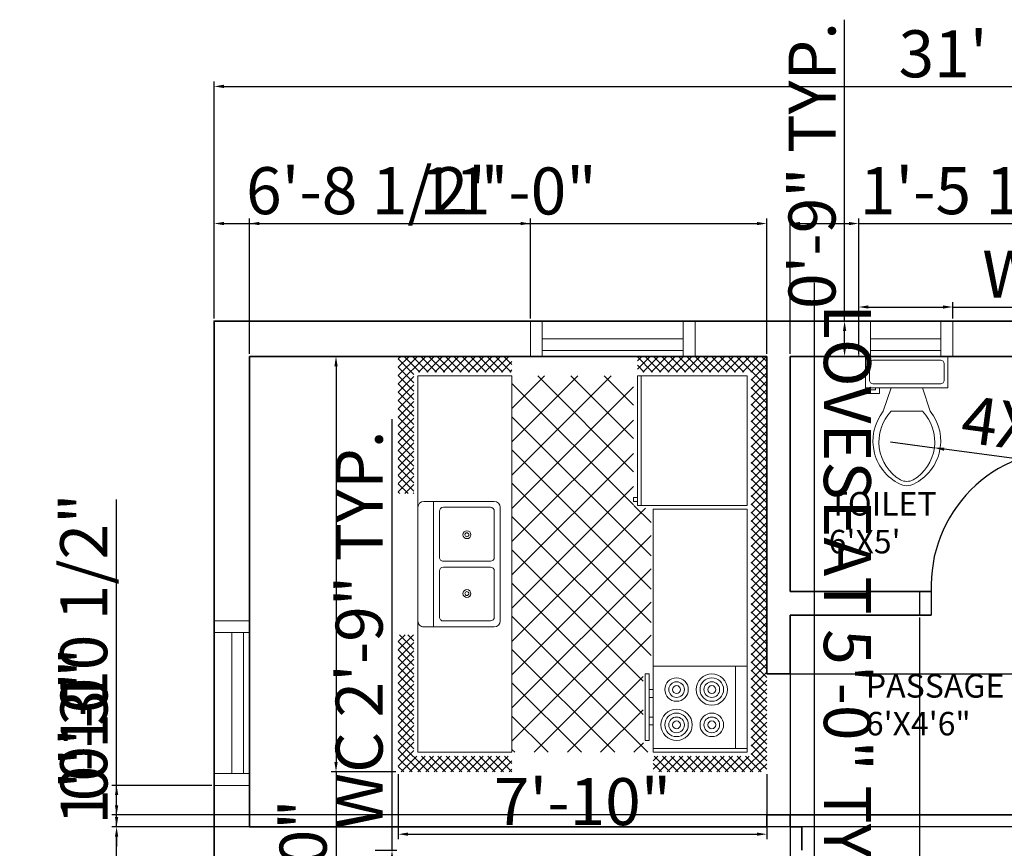
# Model space of a CAD drawing. Units: inches. Extents: x 2330 to 2931, y 514 to 1098.
# Tile 2 of 4: x 2332 to 2583, y 887 to 1098. Entities that reach past the tile are written whole.
import ezdxf

# ---------------------------------------------------------------- set-up
doc = ezdxf.new("R2010")
doc.units = ezdxf.units.IN
for name, color, linetype, lineweight in [('A-ANNO-DIMS', 2, 'Continuous', 18), ('A-AREA-IDEN', 7, 'Continuous', 18), ('A-DOOR', 3, 'Continuous', 25), ('A-FLOR-FIXT', 9, 'Continuous', 18), ('A-GLAZ', 4, 'Continuous', 18), ('A-WALL', 7, 'Continuous', 35)]:
    doc.layers.add(name, color=color, linetype=linetype, lineweight=lineweight)
doc.styles.get("Standard").update_dxf_attribs({"font": 'arial.ttf'})
doc.dimstyles.new('ISO-25', dxfattribs={"dimtxt": 12, "dimasz": 2.5, "dimexe": 1.25, "dimexo": 0.625, "dimtad": 1, "dimdec": 1, "dimlunit": 3, "dimtxsty": 'Standard', "dimcen": 2.5, "dimadec": 0, "dimazin": 0, "dimtfac": 1, "dimtdec": 1, "dimtmove": 0, "dimatfit": 3, "dimfxl": 1, "dimarcsym": 0})

# ---------------------------------------------------------------- blocks, each defined once
blk = doc.blocks.new('*D1')
at = {"layer": 'A-ANNO-DIMS', "color": 0, "lineweight": -2, "transparency": 16777216}
for p, q in [((2381.8, 1022.1), (2381.8, 1082.6)), ((2384.3, 1081.35), (2751.3, 1081.35)), ((2753.8, 1022.1), (2753.8, 1082.6))]:
    blk.add_line(p, q, dxfattribs=at)
at = {"layer": 'A-ANNO-DIMS', "color": 0, "transparency": 16777216}
for points in [[(2384.3, 1081.77), (2384.3, 1080.93), (2381.8, 1081.35)], [(2751.3, 1081.77), (2751.3, 1080.93), (2753.8, 1081.35)]]:
    blk.add_solid(points, dxfattribs=at)
at = {"layer": 'Defpoints', "color": 0, "transparency": 16777216}
for p in [(2753.8, 1081.35), (2381.8, 1021.47), (2753.8, 1021.47)]:
    blk.add_point(p, dxfattribs=at)
at = {"layer": 'A-ANNO-DIMS', "color": 0, "transparency": 16777216, "insert": (2567.8, 1088.11), "char_height": 12, "attachment_point": 5}
blk.add_mtext("31'", dxfattribs=at)
blk = doc.blocks.new('Kitchen Layout - 7 x 8 ft')
for p, q in [((-5, 81.32), (2.68, 89)), ((-5, 83.44), (0.56, 89)), ((-5, 85.56), (-1.56, 89)), ((-5, 87.68), (-3.68, 89)), ((-1, 84.97), (-5, 88.97)), ((1.09, 85), (-2.91, 89)), ((3.21, 85), (-0.79, 89)), ((0.81, 85), (4.81, 89)), ((5.34, 85), (1.34, 89)), ((2.93, 85), (6.93, 89)), ((7.46, 85), (3.46, 89)), ((5.05, 85), (9.05, 89)), ((9.58, 85), (5.58, 89)), ((7.17, 85), (11.17, 89)), ((11.7, 85), (7.7, 89)), ((9.29, 85), (13.29, 89)), ((13.82, 85), (9.82, 89)), ((11.41, 85), (15.41, 89)), ((15.94, 85), (11.94, 89)), ((13.53, 85), (17.53, 89)), ((18.06, 85), (14.06, 89)), ((15.65, 85), (19.65, 89)), ((20.18, 85), (16.18, 89)), ((17.78, 85), (21.78, 89)), ((22.31, 85), (18.31, 89)), ((19.9, 85), (23.9, 89)), ((24.43, 85), (20.43, 89)), ((22.02, 85), (26.02, 89)), ((26.55, 85), (22.55, 89)), ((24.14, 85), (28.14, 89)), ((28.67, 85), (24.67, 89)), ((26.26, 85), (30.26, 89)), ((30.79, 85), (26.79, 89)), ((28.38, 85), (32.38, 89)), ((32.91, 85), (28.91, 89)), ((30.5, 85), (34.5, 89)), ((35.03, 85), (31.03, 89)), ((32.63, 85), (36.63, 89)), ((37.16, 85), (33.16, 89)), ((34.75, 85), (38.75, 89)), ((39.28, 85), (35.28, 89)), ((36.87, 85), (40.87, 89)), ((41.4, 85), (37.4, 89)), ((38.99, 85), (42.99, 89)), ((43.52, 85), (39.52, 89)), ((41.11, 85), (45.11, 89)), ((45.64, 85), (41.64, 89)), ((43.23, 85), (47.23, 89)), ((47.76, 85), (43.76, 89)), ((45.35, 85), (49.35, 89)), ((49.88, 85), (45.88, 89)), ((47.47, 85), (51.47, 89)), ((52, 85), (48, 89)), ((49.6, 85), (53.6, 89)), ((54.13, 85), (50.13, 89)), ((51.72, 85), (55.72, 89)), ((56.25, 85), (52.25, 89)), ((53.84, 85), (57.84, 89)), ((58.37, 85), (54.37, 89)), ((55.96, 85), (59.96, 89)), ((60.49, 85), (56.49, 89)), ((58.08, 85), (62.08, 89)), ((62.61, 85), (58.61, 89)), ((60.2, 85), (64.2, 89)), ((64.73, 85), (60.73, 89)), ((62.32, 85), (66.32, 89)), ((66.85, 85), (62.85, 89)), ((64.45, 85), (68.45, 89)), ((68.97, 85), (64.97, 89)), ((66.57, 85), (70.57, 89)), ((71.1, 85), (67.1, 89)), ((68.69, 85), (72.69, 89)), ((73.22, 85), (69.22, 89)), ((70.81, 85), (74.81, 89)), ((75.34, 85), (71.34, 89)), ((72.93, 85), (76.93, 89)), ((77.46, 85), (73.46, 89)), ((75.05, 85), (79.05, 89)), ((79.58, 85), (75.58, 89)), ((77.17, 85), (81.17, 89)), ((81.7, 85), (77.7, 89)), ((79.29, 85), (83.29, 89)), ((83.82, 85), (79.82, 89)), ((81.42, 85), (85.42, 89)), ((85.95, 85), (81.95, 89)), ((83.54, 85), (87.54, 89)), ((88.07, 85), (84.07, 89)), ((85.66, 85), (89.66, 89)), ((90.19, 85), (86.19, 89)), ((87.78, 85), (91.78, 89)), ((92.31, 85), (88.31, 89)), ((89.9, 85), (93.9, 89)), ((94.43, 85), (90.43, 89)), ((92.02, 85), (96.02, 89)), ((96.55, 85), (92.55, 89)), ((94.14, 85), (98.14, 89)), ((101, 82.67), (94.67, 89)), ((96.27, 85), (100.27, 89)), ((101, 84.79), (96.79, 89)), ((101, 86.92), (98.92, 89)), ((-1, 82.85), (-5, 86.85)), ((97, 83.61), (101, 87.61)), ((97, 81.49), (101, 85.49)), ((-1, 80.73), (-5, 84.73)), ((-5, 79.19), (-1, 83.19)), ((34, 84), (96, 84)), ((34, 60), (34, 84)), ((96, 84), (96, 60)), ((101, 80.55), (97, 84.55)), ((97, 79.37), (101, 83.37)), ((-1, 78.61), (-5, 82.61)), ((-5, 77.07), (-1, 81.07)), ((-1, 76.49), (-5, 80.49)), ((74, 81), (95, 81)), ((101, 78.43), (97, 82.43)), ((97, 77.25), (101, 81.25)), ((-5, 74.95), (-1, 78.95)), ((-1, 74.36), (-5, 78.36)), ((101, 76.31), (97, 80.31)), ((97, 75.13), (101, 79.13)), ((101, 74.19), (97, 78.19)), ((-5, 72.83), (-1, 76.83)), ((-1, 72.24), (-5, 76.24)), ((97, 73.01), (101, 77.01)), ((101, 72.07), (97, 76.07)), ((-5, 70.71), (-1, 74.71)), ((-1, 70.12), (-5, 74.12)), ((97, 70.89), (101, 74.89)), ((101, 69.95), (97, 73.95)), ((-5, 68.59), (-1, 72.59)), ((-1, 68), (-5, 72)), ((-5, 66.47), (-1, 70.47)), ((97, 68.76), (101, 72.76)), ((101, 67.82), (97, 71.82)), ((97, 66.64), (101, 70.64)), ((-1, 65.88), (-5, 69.88)), ((-5, 64.35), (-1, 68.35)), ((101, 65.7), (97, 69.7)), ((97, 64.52), (101, 68.52)), ((-1, 63.76), (-5, 67.76)), ((-5, 62.22), (-1, 66.22)), ((-1, 61.64), (-5, 65.64)), ((101, 63.58), (97, 67.58)), ((97, 62.4), (101, 66.4)), ((101, 61.46), (97, 65.46)), ((-5, 60.1), (-1, 64.1)), ((-1, 59.52), (-5, 63.52)), ((97, 60.28), (101, 64.28)), ((100.34, 60), (97, 63.34)), ((-5, 57.98), (-1, 61.98)), ((-1, 57.39), (-5, 61.39)), ((98.22, 60), (97, 61.22)), ((98.84, 60), (101, 62.16)), ((-1.73, 56), (-5, 59.27)), ((-4.86, 56), (-1, 59.86)), ((10.4, 24), (45.9, 59.5)), ((18.88, 24), (54.38, 59.5)), ((27.37, 24), (62.87, 59.5)), ((33.03, 55.11), (37.41, 59.5)), ((67.71, 24), (33.68, 58.04)), ((96, 60), (34, 60)), ((35.85, 24), (71.35, 59.5)), ((76.2, 24), (40.7, 59.5)), ((84.68, 24), (49.18, 59.5)), ((93.17, 24), (57.67, 59.5)), ((61.31, 24), (96, 58.69)), ((96, 29.65), (66.15, 59.5)), ((80, 60), (80, 59)), ((82, 59), (82, 60)), ((87, 59), (87, 60)), ((89, 60), (89, 59)), ((100.96, 60), (101, 60.04)), ((-3.85, 56), (-5, 57.15)), ((-2.74, 56), (-1, 57.74)), ((0, 57), (33, 57)), ((31, 55), (31, 56)), ((32, 56), (32, 55)), ((44.34, 24), (77.84, 57.5)), ((52.82, 24), (86.32, 57.5)), ((96, 38.14), (76.64, 57.5)), ((96, 46.63), (85.13, 57.5)), ((96, 55.11), (93.57, 57.54)), ((0, 30.57), (24.43, 55)), ((0, 39.06), (15.94, 55)), ((0, 47.54), (7.46, 55)), ((1.91, 24), (32.91, 55)), ((33.77, 24), (2.77, 55)), ((42.26, 24), (11.26, 55)), ((50.74, 24), (19.74, 55)), ((59.23, 24), (28.23, 55)), ((32, 55), (31, 55)), ((25.29, 24), (0, 49.29)), ((69.79, 24), (96, 50.21)), ((16.8, 24), (0, 40.8)), ((78.28, 24), (96, 41.72)), ((86.76, 24), (96, 33.24)), ((8.32, 24), (0, 32.32)), ((-5, 21.92), (-2.92, 24)), ((-5, 19.8), (-1, 23.8)), ((-1, 19.21), (-5, 23.21)), ((-1, 21.33), (-3.67, 24)), ((-1, 23.45), (-1.55, 24)), ((0, 24), (96, 24)), ((0, 0), (0, 24)), ((95.25, 24), (96, 24.75)), ((96, 24), (96, 0)), ((97, 22.1), (98.9, 24)), ((97, 19.97), (101, 23.97)), ((101, 19.03), (97, 23.03)), ((101, 21.16), (98.16, 24)), ((101, 23.28), (100.28, 24)), ((-5, 17.68), (-1, 21.68)), ((-1, 17.09), (-5, 21.09)), ((97, 17.85), (101, 21.85)), ((101, 16.91), (97, 20.91)), ((-5, 15.55), (-1, 19.55)), ((-1, 14.97), (-5, 18.97)), ((47.25, 6.5), (47.25, 18.5)), ((48.75, 18.5), (48.75, 6.5)), ((97, 15.73), (101, 19.73)), ((101, 14.79), (97, 18.79)), ((97, 13.61), (101, 17.61)), ((-5, 13.43), (-1, 17.43)), ((-1, 12.85), (-5, 16.85)), ((-5, 11.31), (-1, 15.31)), ((101, 12.67), (97, 16.67)), ((97, 11.49), (101, 15.49)), ((-1, 10.73), (-5, 14.73)), ((-5, 9.19), (-1, 13.19)), ((-1, 8.6), (-5, 12.6)), ((101, 10.55), (97, 14.55)), ((97, 9.37), (101, 13.37)), ((-5, 7.07), (-1, 11.07)), ((-1, 6.48), (-5, 10.48)), ((101, 8.43), (97, 12.43)), ((97, 7.25), (101, 11.25)), ((101, 6.31), (97, 10.31)), ((-5, 4.95), (-1, 8.95)), ((-1, 4.36), (-5, 8.36)), ((97, 5.12), (101, 9.12)), ((101, 4.18), (97, 8.18)), ((-5, 2.83), (-1, 6.83)), ((-1, 2.24), (-5, 6.24)), ((97, 3), (101, 7)), ((101, 2.06), (97, 6.06)), ((-5, 0.71), (-1, 4.71)), ((-1, 0.12), (-5, 4.12)), ((-5, -1.42), (-1, 2.58)), ((64, 4), (32, 4)), ((93.24, -5), (101, 2.76)), ((97, 0.88), (101, 4.88)), ((101, -0.06), (97, 3.94)), ((2, -5), (-5, 2)), ((-5, -3.54), (-1, 0.46)), ((96, 0), (0, 0)), ((95.36, -5), (101, 0.64)), ((101, -2.18), (97, 1.82)), ((-0.12, -5), (-5, -0.12)), ((-2.25, -5), (-5, -2.25)), ((-4.34, -5), (-0.34, -1)), ((-2.22, -5), (1.78, -1)), ((-0.1, -5), (3.9, -1)), ((4.12, -5), (0.12, -1)), ((2.02, -5), (6.02, -1)), ((6.24, -5), (2.24, -1)), ((4.14, -5), (8.14, -1)), ((8.36, -5), (4.36, -1)), ((6.27, -5), (10.27, -1)), ((10.48, -5), (6.48, -1)), ((8.39, -5), (12.39, -1)), ((12.6, -5), (8.6, -1)), ((10.51, -5), (14.51, -1)), ((14.73, -5), (10.73, -1)), ((12.63, -5), (16.63, -1)), ((16.85, -5), (12.85, -1)), ((14.75, -5), (18.75, -1)), ((18.97, -5), (14.97, -1)), ((16.87, -5), (20.87, -1)), ((21.09, -5), (17.09, -1)), ((18.99, -5), (22.99, -1)), ((23.21, -5), (19.21, -1)), ((21.11, -5), (25.11, -1)), ((25.33, -5), (21.33, -1)), ((23.24, -5), (27.24, -1)), ((27.45, -5), (23.45, -1)), ((25.36, -5), (29.36, -1)), ((29.57, -5), (25.57, -1)), ((27.48, -5), (30, -2.48)), ((30, -3.3), (27.7, -1)), ((30, -1.18), (29.82, -1)), ((66, -2.54), (67.54, -1)), ((66, -4.66), (69.66, -1)), ((69.88, -5), (66, -1.12)), ((67.78, -5), (71.78, -1)), ((72, -5), (68, -1)), ((69.9, -5), (73.9, -1)), ((74.12, -5), (70.12, -1)), ((72.03, -5), (76.03, -1)), ((76.24, -5), (72.24, -1)), ((74.15, -5), (78.15, -1)), ((78.36, -5), (74.36, -1)), ((76.27, -5), (80.27, -1)), ((80.49, -5), (76.49, -1)), ((78.39, -5), (82.39, -1)), ((82.61, -5), (78.61, -1)), ((80.51, -5), (84.51, -1)), ((84.73, -5), (80.73, -1)), ((82.63, -5), (86.63, -1)), ((86.85, -5), (82.85, -1)), ((84.75, -5), (88.75, -1)), ((88.97, -5), (84.97, -1)), ((86.88, -5), (90.88, -1)), ((91.09, -5), (87.09, -1)), ((89, -5), (93, -1)), ((93.21, -5), (89.21, -1)), ((91.12, -5), (95.12, -1)), ((95.34, -5), (91.34, -1)), ((97.46, -5), (93.46, -1)), ((99.58, -5), (95.58, -1)), ((101, -4.3), (97, -0.3)), ((97.48, -5), (101, -1.48)), ((-4.37, -5), (-5, -4.37)), ((29.6, -5), (30, -4.6)), ((67.76, -5), (66, -3.24)), ((99.6, -5), (101, -3.6))]:
    blk.add_line(p, q)
for points in [[(0, 56), (0, 84), (33, 84), (33, 56)], [(74, 60), (74, 84), (95, 84), (95, 60)], [(76, 58), (76, 59), (93, 59), (93, 58)]]:
    blk.add_lwpolyline(points, close=True)
for points in [[(33.5, 21), (62.5, 21)], [(32, 1.5), (32, 19.5)], [(33.5, 6.5), (33.5, 18.5)], [(34.5, 19.5), (46.25, 19.5)], [(49.75, 19.5), (61.5, 19.5)], [(62.5, 18.5), (62.5, 6.5)], [(64, 19.5), (64, 1.5)], [(46.25, 5.5), (34.5, 5.5)], [(61.5, 5.5), (49.75, 5.5)], [(62.5, 0), (33.5, 0)]]:
    blk.add_lwpolyline(points)
for centre, radius in [((80, 75), 4), ((80, 75), 3), ((89, 75), 3), ((80, 75), 2), ((80, 75), 1), ((89, 75), 2), ((89, 75), 1), ((80, 66), 3), ((80, 66), 2), ((89, 66), 4), ((89, 66), 3), ((89, 66), 2), ((80, 66), 1), ((89, 66), 1), ((40.5, 12.5), 1), ((40.5, 12.5), 0.5), ((55.5, 12.5), 1), ((55.5, 12.5), 0.5)]:
    blk.add_circle(centre, radius)
for centre, radius, start, end in [((33.5, 19.5), 1.5, 90, 180), ((62.5, 19.5), 1.5, 0, 90), ((34.5, 18.5), 1, 90, 180), ((46.25, 18.5), 1, 0, 90), ((49.75, 18.5), 1, 90, 180), ((61.5, 18.5), 1, 0, 90), ((34.5, 6.5), 1, 180, 270), ((46.25, 6.5), 1, 270, 0), ((49.75, 6.5), 1, 180, 270), ((61.5, 6.5), 1, 270, 0), ((33.5, 1.5), 1.5, 180, 270), ((62.5, 1.5), 1.5, 270, 0)]:
    blk.add_arc(centre, radius, start, end)
blk = doc.blocks.new('Toilet - top')
for p, q in [((9.5, -6), (9.5, -2)), ((-10, -8.5), (-8, -8.5)), ((-10, -9.5), (-10, -8.5)), ((-7, -9.5), (-10, -9.5)), ((-8, -8.5), (-8, -8)), ((-7, -8), (-7, -9.5)), ((-4, -8), (-6, -14)), ((4, -8), (6, -14)), ((4, -14), (-4, -14))]:
    blk.add_line(p, q)
blk.add_lwpolyline([(10.5, -8), (10.5, 0), (-10.5, 0), (-10.5, -8)], close=True)
for points in [[(-9.5, -2), (-9.5, -6)], [(8.5, -1), (-8.5, -1)], [(-8.5, -7), (8.5, -7)]]:
    blk.add_lwpolyline(points)
for centre, radius, start, end in [((-8.62, -1.88), 0.884, 81.8699, 188.1301), ((8.62, -1.88), 0.884, 351.8699, 98.1301), ((-8.62, -6.12), 0.884, 171.8699, 278.1301), ((8.62, -6.12), 0.884, 261.8699, 8.1301), ((3.52, -21.58), 12.17, 141.4691, 247.9714), ((4.2, -21.82), 11.33, 136.3677, 238.9468), ((-3.52, -21.58), 12.17, 292.0284, 38.5307), ((-4.2, -21.82), 11.33, 301.053, 43.6321), ((0, -27.88), 4, 245.7318, 294.2682), ((0, -29), 4, 254.8605, 285.1395)]:
    blk.add_arc(centre, radius, start, end)
blk = doc.blocks.new('DOOR-SWING-36IN')
for p, q in [((0, 6), (0, 0)), ((3, 6), (3, 0)), ((39, 6), (39, 0)), ((42, 6), (42, 0))]:
    blk.add_line(p, q)
blk.add_lwpolyline([(39, 6), (36, 6), (36, 42), (39, 42)], close=True)
blk.add_arc((37.5, 7.5), 34.53, 87.5104, 182.4896)
blk = doc.blocks.new('WIN-36IN')
for p, q in [((0, 9), (0, 0)), ((39, 9), (3, 9)), ((3, 9), (3, 0)), ((39, 0), (39, 9)), ((42, 0), (42, 9)), ((3, 4.5), (39, 4.5)), ((3, 1.5), (39, 1.5)), ((3, 0), (39, 0))]:
    blk.add_line(p, q)
blk = doc.blocks.new('WIN-18IN')
for p, q in [((0, 9), (0, 0)), ((21, 9), (3, 9)), ((3, 9), (3, 0)), ((21, 0), (21, 9)), ((24, 0), (24, 9)), ((3, 4.5), (21, 4.5)), ((3, 1.5), (21, 1.5)), ((3, 0), (21, 0))]:
    blk.add_line(p, q)
blk = doc.blocks.new('*D19')
at = {"layer": 'A-ANNO-DIMS', "color": 0, "lineweight": -2, "transparency": 16777216}
for p, q in [((2546.27, 1022.1), (2546.27, 1026.32)), ((2570.27, 1022.1), (2570.27, 1026.32)), ((2548.77, 1025.07), (2567.77, 1025.07)), ((2570.27, 1025.07), (2755.68, 1025.07))]:
    blk.add_line(p, q, dxfattribs=at)
at = {"layer": 'A-ANNO-DIMS', "color": 0, "transparency": 16777216}
for points in [[(2548.77, 1025.49), (2548.77, 1024.66), (2546.27, 1025.07)], [(2567.77, 1025.49), (2567.77, 1024.66), (2570.27, 1025.07)]]:
    blk.add_solid(points, dxfattribs=at)
at = {"layer": 'Defpoints', "color": 0, "transparency": 16777216}
for p in [(2570.27, 1025.07), (2546.27, 1021.47), (2570.27, 1021.47)]:
    blk.add_point(p, dxfattribs=at)
at = {"layer": 'A-ANNO-DIMS', "color": 0, "transparency": 16777216, "insert": (2664.23, 1031.91), "char_height": 12, "attachment_point": 5}
blk.add_mtext('WINDOW W2 2\'-0" TYP.', dxfattribs=at)
blk = doc.blocks.new('*D20')
at = {"layer": 'A-ANNO-DIMS', "color": 0, "lineweight": -2, "transparency": 16777216}
for p, q in [((2542.67, 1021.47), (2542.67, 1098.37)), ((2545.65, 1021.47), (2541.42, 1021.47)), ((2542.67, 1014.97), (2542.67, 1018.97)), ((2545.65, 1012.47), (2541.42, 1012.47))]:
    blk.add_line(p, q, dxfattribs=at)
at = {"layer": 'A-ANNO-DIMS', "color": 0, "transparency": 16777216}
for points in [[(2542.26, 1018.97), (2543.09, 1018.97), (2542.67, 1021.47)], [(2542.26, 1014.97), (2543.09, 1014.97), (2542.67, 1012.47)]]:
    blk.add_solid(points, dxfattribs=at)
at = {"layer": 'Defpoints', "color": 0, "transparency": 16777216}
for p in [(2542.67, 1021.47), (2546.27, 1021.47), (2546.27, 1012.47)]:
    blk.add_point(p, dxfattribs=at)
at = {"layer": 'A-ANNO-DIMS', "color": 0, "transparency": 16777216, "insert": (2535.92, 1061.17), "char_height": 12, "attachment_point": 5, "rotation": 90}
blk.add_mtext('0\'-9" TYP.', dxfattribs=at)
blk = doc.blocks.new('*D23')
at = {"layer": 'A-ANNO-DIMS', "color": 0, "lineweight": -2, "transparency": 16777216}
for p, q in [((2427.19, 886.47), (2427.19, 996.45)), ((2422.86, 886.47), (2428.44, 886.47)), ((2427.19, 855.93), (2427.19, 883.97)), ((2422.86, 853.43), (2428.44, 853.43))]:
    blk.add_line(p, q, dxfattribs=at)
at = {"layer": 'A-ANNO-DIMS', "color": 0, "transparency": 16777216}
for points in [[(2426.77, 883.97), (2427.61, 883.97), (2427.19, 886.47)], [(2426.77, 855.93), (2427.61, 855.93), (2427.19, 853.43)]]:
    blk.add_solid(points, dxfattribs=at)
at = {"layer": 'Defpoints', "color": 0, "transparency": 16777216}
for p in [(2422.23, 886.47), (2427.19, 886.47), (2422.23, 853.43)]:
    blk.add_point(p, dxfattribs=at)
at = {"layer": 'A-ANNO-DIMS', "color": 0, "transparency": 16777216, "insert": (2420.36, 942.71), "char_height": 12, "attachment_point": 5, "rotation": 90}
blk.add_mtext('WC 2\'-9" TYP.', dxfattribs=at)
blk = doc.blocks.new('*D25')
at = {"layer": 'A-ANNO-DIMS', "color": 0, "lineweight": -2, "transparency": 16777216}
for p, q in [((2535, 861.7), (2535, 1031.23)), ((2543.37, 861.7), (2533.75, 861.7)), ((2535, 804.2), (2535, 859.2)), ((2543.37, 801.7), (2533.75, 801.7))]:
    blk.add_line(p, q, dxfattribs=at)
at = {"layer": 'A-ANNO-DIMS', "color": 0, "transparency": 16777216}
for points in [[(2535.41, 859.2), (2534.58, 859.2), (2535, 861.7)], [(2535.41, 804.2), (2534.58, 804.2), (2535, 801.7)]]:
    blk.add_solid(points, dxfattribs=at)
at = {"layer": 'Defpoints', "color": 0, "transparency": 16777216}
for p in [(2535, 861.7), (2544, 861.7), (2544, 801.7)]:
    blk.add_point(p, dxfattribs=at)
at = {"layer": 'A-ANNO-DIMS', "color": 0, "transparency": 16777216, "insert": (2541.83, 947.72), "char_height": 12, "attachment_point": 5, "rotation": 270.0001}
blk.add_mtext('LOVESEAT 5\'-0" TYP.', dxfattribs=at)
blk = doc.blocks.new('*D31')
at = {"layer": 'A-ANNO-DIMS', "color": 0, "lineweight": -2, "transparency": 16777216}
for p, q in [((2428.18, 1012.47), (2411.65, 1012.47)), ((2412.9, 1009.97), (2412.9, 908.97)), ((2428.18, 906.47), (2411.65, 906.47)), ((2412.9, 906.47), (2412.9, 712.06))]:
    blk.add_line(p, q, dxfattribs=at)
at = {"layer": 'A-ANNO-DIMS', "color": 0, "transparency": 16777216}
for points in [[(2412.49, 1009.97), (2413.32, 1009.97), (2412.9, 1012.47)], [(2412.49, 908.97), (2413.32, 908.97), (2412.9, 906.47)]]:
    blk.add_solid(points, dxfattribs=at)
at = {"layer": 'Defpoints', "color": 0, "transparency": 16777216}
for p in [(2428.8, 1012.47), (2412.9, 906.47), (2428.8, 906.47)]:
    blk.add_point(p, dxfattribs=at)
at = {"layer": 'A-ANNO-DIMS', "color": 0, "transparency": 16777216, "insert": (2406.07, 808.02), "char_height": 12, "attachment_point": 5, "rotation": 90}
blk.add_mtext('KITCHEN LAYOUT 8\'-10"', dxfattribs=at)
blk = doc.blocks.new('*D32')
at = {"layer": 'A-ANNO-DIMS', "color": 0, "lineweight": -2, "transparency": 16777216}
for p, q in [((2428.8, 905.85), (2428.8, 889.32)), ((2522.8, 905.85), (2522.8, 889.32)), ((2431.3, 890.57), (2520.3, 890.57))]:
    blk.add_line(p, q, dxfattribs=at)
at = {"layer": 'A-ANNO-DIMS', "color": 0, "transparency": 16777216}
for points in [[(2431.3, 890.99), (2431.3, 890.16), (2428.8, 890.57)], [(2520.3, 890.99), (2520.3, 890.16), (2522.8, 890.57)]]:
    blk.add_solid(points, dxfattribs=at)
at = {"layer": 'Defpoints', "color": 0, "transparency": 16777216}
for p in [(2428.8, 906.47), (2522.8, 906.47), (2522.8, 890.57)]:
    blk.add_point(p, dxfattribs=at)
at = {"layer": 'A-ANNO-DIMS', "color": 0, "transparency": 16777216, "insert": (2475.8, 897.32), "char_height": 12, "attachment_point": 5}
blk.add_mtext('7\'-10"', dxfattribs=at)
blk = doc.blocks.new('*D37')
at = {"layer": 'A-ANNO-DIMS', "color": 0, "lineweight": -2, "transparency": 16777216}
for p, q in [((2390.8, 1013.1), (2390.8, 1047.61)), ((2393.3, 1046.36), (2520.3, 1046.36)), ((2522.8, 1013.1), (2522.8, 1047.61))]:
    blk.add_line(p, q, dxfattribs=at)
at = {"layer": 'A-ANNO-DIMS', "color": 0, "transparency": 16777216}
for points in [[(2393.3, 1046.78), (2393.3, 1045.95), (2390.8, 1046.36)], [(2520.3, 1046.78), (2520.3, 1045.95), (2522.8, 1046.36)]]:
    blk.add_solid(points, dxfattribs=at)
at = {"layer": 'Defpoints', "color": 0, "transparency": 16777216}
for p in [(2522.8, 1046.36), (2390.8, 1012.47), (2522.8, 1012.47)]:
    blk.add_point(p, dxfattribs=at)
at = {"layer": 'A-ANNO-DIMS', "color": 0, "transparency": 16777216, "insert": (2456.8, 1053.12), "char_height": 12, "attachment_point": 5}
blk.add_mtext('11\'-0"', dxfattribs=at)
blk = doc.blocks.new('*D38')
at = {"layer": 'A-ANNO-DIMS', "color": 0, "lineweight": -2, "transparency": 16777216}
for p, q in [((2381.8, 1022.1), (2381.8, 1047.61)), ((2384.3, 1046.36), (2460.01, 1046.36)), ((2462.51, 1022.1), (2462.51, 1047.61))]:
    blk.add_line(p, q, dxfattribs=at)
at = {"layer": 'A-ANNO-DIMS', "color": 0, "transparency": 16777216}
for points in [[(2384.3, 1046.78), (2384.3, 1045.95), (2381.8, 1046.36)], [(2460.01, 1046.78), (2460.01, 1045.95), (2462.51, 1046.36)]]:
    blk.add_solid(points, dxfattribs=at)
at = {"layer": 'Defpoints', "color": 0, "transparency": 16777216}
for p in [(2462.51, 1046.36), (2381.8, 1021.47), (2462.51, 1021.47)]:
    blk.add_point(p, dxfattribs=at)
at = {"layer": 'A-ANNO-DIMS', "color": 0, "transparency": 16777216, "insert": (2422.16, 1053.19), "char_height": 12, "attachment_point": 5}
blk.add_mtext('6\'-8 1/2"', dxfattribs=at)
blk = doc.blocks.new('*D40')
at = {"layer": 'A-ANNO-DIMS', "color": 0, "lineweight": -2, "transparency": 16777216}
for p, q in [((2528.8, 1013.1), (2528.8, 1047.61)), ((2531.3, 1046.36), (2543.77, 1046.36)), ((2546.27, 1013.1), (2546.27, 1047.61)), ((2546.27, 1046.36), (2608.76, 1046.36))]:
    blk.add_line(p, q, dxfattribs=at)
at = {"layer": 'A-ANNO-DIMS', "color": 0, "transparency": 16777216}
for points in [[(2531.3, 1046.78), (2531.3, 1045.95), (2528.8, 1046.36)], [(2543.77, 1046.78), (2543.77, 1045.95), (2546.27, 1046.36)]]:
    blk.add_solid(points, dxfattribs=at)
at = {"layer": 'Defpoints', "color": 0, "transparency": 16777216}
for p in [(2546.27, 1046.36), (2528.8, 1012.47), (2546.27, 1012.47)]:
    blk.add_point(p, dxfattribs=at)
at = {"layer": 'A-ANNO-DIMS', "color": 0, "transparency": 16777216, "insert": (2578.76, 1053.19), "char_height": 12, "attachment_point": 5}
blk.add_mtext('1\'-5 1/2"', dxfattribs=at)
blk = doc.blocks.new('*D44')
at = {"layer": 'A-ANNO-DIMS', "color": 0, "lineweight": -2, "transparency": 16777216}
for p, q in [((2356.91, 892.47), (2356.91, 936.31)), ((2390.18, 892.47), (2355.66, 892.47)), ((2356.91, 872.73), (2356.91, 889.97)), ((2381.18, 870.23), (2355.66, 870.23))]:
    blk.add_line(p, q, dxfattribs=at)
at = {"layer": 'A-ANNO-DIMS', "color": 0, "transparency": 16777216}
for points in [[(2356.49, 889.97), (2357.33, 889.97), (2356.91, 892.47)], [(2356.49, 872.73), (2357.33, 872.73), (2356.91, 870.23)]]:
    blk.add_solid(points, dxfattribs=at)
at = {"layer": 'Defpoints', "color": 0, "transparency": 16777216}
for p in [(2356.91, 892.47), (2390.8, 892.47), (2381.8, 870.23)]:
    blk.add_point(p, dxfattribs=at)
at = {"layer": 'A-ANNO-DIMS', "color": 0, "transparency": 16777216, "insert": (2350.16, 915.64), "char_height": 12, "attachment_point": 5, "rotation": 90}
blk.add_mtext('1\'-10"', dxfattribs=at)
blk = doc.blocks.new('*D45')
at = {"layer": 'A-ANNO-DIMS', "color": 0, "lineweight": -2, "transparency": 16777216}
for p, q in [((2356.91, 903.03), (2356.91, 975.96)), ((2381.18, 903.03), (2355.66, 903.03)), ((2356.91, 894.97), (2356.91, 900.53)), ((2390.18, 892.47), (2355.66, 892.47))]:
    blk.add_line(p, q, dxfattribs=at)
at = {"layer": 'A-ANNO-DIMS', "color": 0, "transparency": 16777216}
for points in [[(2356.49, 900.53), (2357.33, 900.53), (2356.91, 903.03)], [(2356.49, 894.97), (2357.33, 894.97), (2356.91, 892.47)]]:
    blk.add_solid(points, dxfattribs=at)
at = {"layer": 'Defpoints', "color": 0, "transparency": 16777216}
for p in [(2356.91, 903.03), (2381.8, 903.03), (2390.8, 892.47)]:
    blk.add_point(p, dxfattribs=at)
at = {"layer": 'A-ANNO-DIMS', "color": 0, "transparency": 16777216, "insert": (2350.08, 940.74), "char_height": 12, "attachment_point": 5, "rotation": 90}
blk.add_mtext('0\'-10 1/2"', dxfattribs=at)
blk = doc.blocks.new('*D53')
at = {"layer": 'A-ANNO-DIMS', "color": 0, "lineweight": -2, "transparency": 16777216}
for p, q in [((2523.43, 931.47), (2779.95, 931.47)), ((2778.7, 897.97), (2778.7, 928.97)), ((2523.43, 895.47), (2779.95, 895.47))]:
    blk.add_line(p, q, dxfattribs=at)
at = {"layer": 'A-ANNO-DIMS', "color": 0, "transparency": 16777216}
for points in [[(2778.28, 928.97), (2779.11, 928.97), (2778.7, 931.47)], [(2778.28, 897.97), (2779.11, 897.97), (2778.7, 895.47)]]:
    blk.add_solid(points, dxfattribs=at)
at = {"layer": 'Defpoints', "color": 0, "transparency": 16777216}
for p in [(2522.8, 931.47), (2778.7, 931.47), (2522.8, 895.47)]:
    blk.add_point(p, dxfattribs=at)
at = {"layer": 'A-ANNO-DIMS', "color": 0, "transparency": 16777216, "insert": (2771.94, 913.47), "char_height": 12, "attachment_point": 5, "rotation": 90}
blk.add_mtext('3\'-0"', dxfattribs=at)
blk = doc.blocks.new('*D56')
at = {"layer": 'A-ANNO-DIMS', "color": 0, "lineweight": -2, "transparency": 16777216}
for p, q in [((2528.8, 945.85), (2528.8, 572.33)), ((2561.8, 945.85), (2561.8, 572.33)), ((2531.3, 573.58), (2559.3, 573.58)), ((2561.8, 573.58), (2597.66, 573.58))]:
    blk.add_line(p, q, dxfattribs=at)
at = {"layer": 'A-ANNO-DIMS', "color": 0, "transparency": 16777216}
for points in [[(2531.3, 574), (2531.3, 573.16), (2528.8, 573.58)], [(2559.3, 574), (2559.3, 573.16), (2561.8, 573.58)]]:
    blk.add_solid(points, dxfattribs=at)
at = {"layer": 'Defpoints', "color": 0, "transparency": 16777216}
for p in [(2528.8, 946.47), (2561.8, 946.47), (2561.8, 573.58)]:
    blk.add_point(p, dxfattribs=at)
at = {"layer": 'A-ANNO-DIMS', "color": 0, "transparency": 16777216, "insert": (2580.98, 580.33), "char_height": 12, "attachment_point": 5}
blk.add_mtext('2\'-9"', dxfattribs=at)
blk = doc.blocks.new('*D57')
at = {"layer": 'A-ANNO-DIMS', "color": 0, "lineweight": -2, "transparency": 16777216}
for p, q in [((2356.91, 897.97), (2356.91, 933.62)), ((2612.18, 895.47), (2355.66, 895.47)), ((2356.91, 892.47), (2356.91, 895.47)), ((2612.18, 892.47), (2355.66, 892.47)), ((2356.91, 889.97), (2356.91, 887.47))]:
    blk.add_line(p, q, dxfattribs=at)
at = {"layer": 'A-ANNO-DIMS', "color": 0, "transparency": 16777216}
for points in [[(2356.49, 897.97), (2357.33, 897.97), (2356.91, 895.47)], [(2356.49, 889.97), (2357.33, 889.97), (2356.91, 892.47)]]:
    blk.add_solid(points, dxfattribs=at)
at = {"layer": 'Defpoints', "color": 0, "transparency": 16777216}
for p in [(2356.91, 895.47), (2612.8, 895.47), (2612.8, 892.47)]:
    blk.add_point(p, dxfattribs=at)
at = {"layer": 'A-ANNO-DIMS', "color": 0, "transparency": 16777216, "insert": (2350.15, 917.05), "char_height": 12, "attachment_point": 5, "rotation": 90}
blk.add_mtext('0\'-3"', dxfattribs=at)
blk = doc.blocks.new('*D64')
at = {"layer": 'A-ANNO-DIMS', "color": 0, "lineweight": -2, "transparency": 16777216}
for p, q in [((2554.35, 990.65), (2565.58, 989.14)), ((2677.75, 974.06), (2568.05, 988.81))]:
    blk.add_line(p, q, dxfattribs=at)
at = {"layer": 'A-ANNO-DIMS', "color": 0, "transparency": 16777216}
blk.add_solid([(2568.11, 989.22), (2568, 988.4), (2565.58, 989.14)], dxfattribs=at)
at = {"layer": 'Defpoints', "color": 0, "transparency": 16777216}
for p in [(2554.35, 990.65), (2565.58, 989.14)]:
    blk.add_point(p, dxfattribs=at)
at = {"layer": 'A-ANNO-DIMS', "color": 0, "transparency": 16777216, "insert": (2625.05, 988.04), "char_height": 12, "attachment_point": 5, "rotation": 352.3416}
blk.add_mtext('4X R0\'-11 1/2"', dxfattribs=at)

msp = doc.modelspace()

# ---------------------------------------------------------------- linework, layer by layer
at = {"layer": 'A-WALL'}
for p, q in [((2390.8, 1012.47), (2390.8, 892.47)), ((2522.8, 1012.47), (2390.8, 1012.47)), ((2522.8, 1012.47), (2522.8, 931.47)), ((2522.8, 1012.47), (2522.8, 931.47)), ((2528.8, 1012.47), (2528.8, 952.47)), ((2606.8, 1012.47), (2528.8, 1012.47)), ((2564.8, 952.47), (2528.8, 952.47)), ((2528.8, 946.47), (2528.8, 931.47)), ((2564.8, 946.47), (2528.8, 946.47)), ((2522.8, 931.47), (2528.8, 931.47)), ((2522.8, 895.47), (2528.8, 895.47)), ((2522.8, 895.47), (2522.8, 892.47)), ((2522.8, 895.47), (2522.8, 892.47)), ((2528.8, 895.47), (2528.8, 892.47)), ((2522.8, 892.47), (2390.8, 892.47)), ((2531.8, 892.47), (2528.8, 892.47)), ((2531.8, 892.47), (2531.8, 886.47))]:
    msp.add_line(p, q, dxfattribs=at)
msp.add_lwpolyline([(2738.8, 598.47), (2753.8, 598.47), (2753.8, 1021.47), (2381.8, 1021.47), (2381.8, 598.47), (2624.83, 598.47)], dxfattribs=at)

# ---------------------------------------------------------------- block references
at = {"layer": 'A-DOOR'}
msp.add_blockref('DOOR-SWING-36IN', (2561.8, 946.47), dxfattribs=at)
at = {"layer": 'A-FLOR-FIXT', "rotation": 270}
msp.add_blockref('Kitchen Layout - 7 x 8 ft', (2433.8, 1007.47), dxfattribs=at)
at = {"layer": 'A-FLOR-FIXT'}
msp.add_blockref('Toilet - top', (2558.55, 1012.47), dxfattribs=at)
at = {"layer": 'A-GLAZ'}
for name, p in [('WIN-36IN', (2462.51, 1012.47)), ('WIN-18IN', (2546.27, 1012.47))]:
    msp.add_blockref(name, p, dxfattribs=at)
at = {"layer": 'A-GLAZ', "rotation": 89.99999999999976}
msp.add_blockref('WIN-36IN', (2390.8, 903.03), dxfattribs=at)

# ---------------------------------------------------------------- texts
at = {"layer": 'A-AREA-IDEN'}
for s, p in [('TOILET', (2538.62, 971.86)), ("6'X5'", (2538.62, 962.22)), ('PASSAGE', (2548.1, 925.41)), ('6\'X4\'6"', (2548.1, 915.77))]:
    msp.add_text(s, height=6, dxfattribs=at).set_placement(p)

# ---------------------------------------------------------------- dimensions: what is measured, and where the dimension line sits
at = {"layer": 'A-ANNO-DIMS'}
for base, p1, p2, angle, text, picture, middle in [((2542.67, 1021.47), (2546.27, 1012.47), (2546.27, 1021.47), 90, '<> TYP.', '*D20', (2535.92, 1061.17)), ((2535, 861.7), (2544, 801.7), (2544, 861.7), 90.0001, 'LOVESEAT <> TYP.', '*D25', (2541.83, 947.72)), ((2412.9, 906.47), (2428.8, 1012.47), (2428.8, 906.47), 270, 'KITCHEN LAYOUT <>', '*D31', (2406.07, 808.02)), ((2427.19, 886.47), (2422.23, 853.43), (2422.23, 886.47), 90, 'WC <> TYP.', '*D23', (2420.36, 942.71))]:
    dim = msp.add_linear_dim(base=base, p1=p1, p2=p2, angle=angle, text=text, dimstyle='ISO-25', override={"dimdec": 1, "dimlfac": 1, "dimrnd": 0, "dimzin": 1, "dimdsep": 46, "dimlunit": 4, "dimfrac": 2}, dxfattribs=at)
    dim.commit()
    dim.dimension.update_dxf_attribs({"geometry": picture, "text_midpoint": middle})
for base, p1, p2, override, picture, middle in [((2753.8, 1081.35), (2381.8, 1021.47), (2753.8, 1021.47), {"dimclrd": 0, "dimclre": 0, "dimclrt": 0}, '*D1', (2567.8, 1088.11)), ((2462.51, 1046.36), (2381.8, 1021.47), (2462.51, 1021.47), {"dimdec": 1, "dimlfac": 1, "dimrnd": 0, "dimzin": 1, "dimdsep": 46, "dimlunit": 4, "dimfrac": 2}, '*D38', (2422.16, 1053.19)), ((2546.27, 1046.36), (2528.8, 1012.47), (2546.27, 1012.47), {"dimdec": 1, "dimlfac": 1, "dimrnd": 0, "dimzin": 1, "dimdsep": 46, "dimlunit": 4, "dimfrac": 2}, '*D40', (2578.76, 1053.19)), ((2522.8, 1046.36), (2390.8, 1012.47), (2522.8, 1012.47), {"dimdec": 1, "dimlfac": 1, "dimrnd": 0, "dimzin": 1, "dimdsep": 46, "dimlunit": 4, "dimfrac": 2}, '*D37', (2456.8, 1053.12)), ((2561.8, 573.58), (2528.8, 946.47), (2561.8, 946.47), {"dimdec": 1, "dimlfac": 1, "dimrnd": 0, "dimzin": 1, "dimdsep": 46, "dimlunit": 4, "dimfrac": 2}, '*D56', (2580.98, 580.33)), ((2522.8, 890.57), (2428.8, 906.47), (2522.8, 906.47), {"dimdec": 1, "dimlfac": 1, "dimrnd": 0, "dimzin": 1, "dimdsep": 46, "dimlunit": 4, "dimfrac": 2}, '*D32', (2475.8, 897.32))]:
    dim = msp.add_linear_dim(base=base, p1=p1, p2=p2, dimstyle='ISO-25', override=override, dxfattribs=at)
    dim.commit()
    dim.dimension.update_dxf_attribs({"geometry": picture, "text_midpoint": middle})
dim = msp.add_linear_dim(base=(2570.27, 1025.07), p1=(2546.27, 1021.47), p2=(2570.27, 1021.47), text='WINDOW W2 <> TYP.', dimstyle='ISO-25', override={"dimdec": 1, "dimlfac": 1, "dimrnd": 0, "dimzin": 1, "dimdsep": 46, "dimlunit": 4, "dimfrac": 2}, dxfattribs=at)
dim.commit()
dim.dimension.update_dxf_attribs({"geometry": '*D19', "text_midpoint": (2664.23, 1031.91)})
dim = msp.add_radius_dim(center=(2554.35, 990.65), mpoint=(2565.58, 989.14), text='4X <>', dimstyle='ISO-25', override={"dimdec": 1, "dimlfac": 1, "dimrnd": 0, "dimzin": 1, "dimdsep": 46, "dimlunit": 4, "dimfrac": 2}, dxfattribs=at)
dim.commit()
dim.dimension.update_dxf_attribs({"geometry": '*D64', "text_midpoint": (2625.05, 988.04)})
for base, p1, p2, picture, middle in [((2356.91, 903.03), (2390.8, 892.47), (2381.8, 903.03), '*D45', (2350.08, 940.74)), ((2356.91, 892.47), (2381.8, 870.23), (2390.8, 892.47), '*D44', (2350.16, 915.64)), ((2356.91, 895.47), (2612.8, 892.47), (2612.8, 895.47), '*D57', (2350.15, 917.05)), ((2778.7, 931.47), (2522.8, 895.47), (2522.8, 931.47), '*D53', (2771.94, 913.47))]:
    dim = msp.add_linear_dim(base=base, p1=p1, p2=p2, angle=90, dimstyle='ISO-25', override={"dimdec": 1, "dimlfac": 1, "dimrnd": 0, "dimzin": 1, "dimdsep": 46, "dimlunit": 4, "dimfrac": 2}, dxfattribs=at)
    dim.commit()
    dim.dimension.update_dxf_attribs({"geometry": picture, "text_midpoint": middle})

doc.saveas('drawing.dxf')
